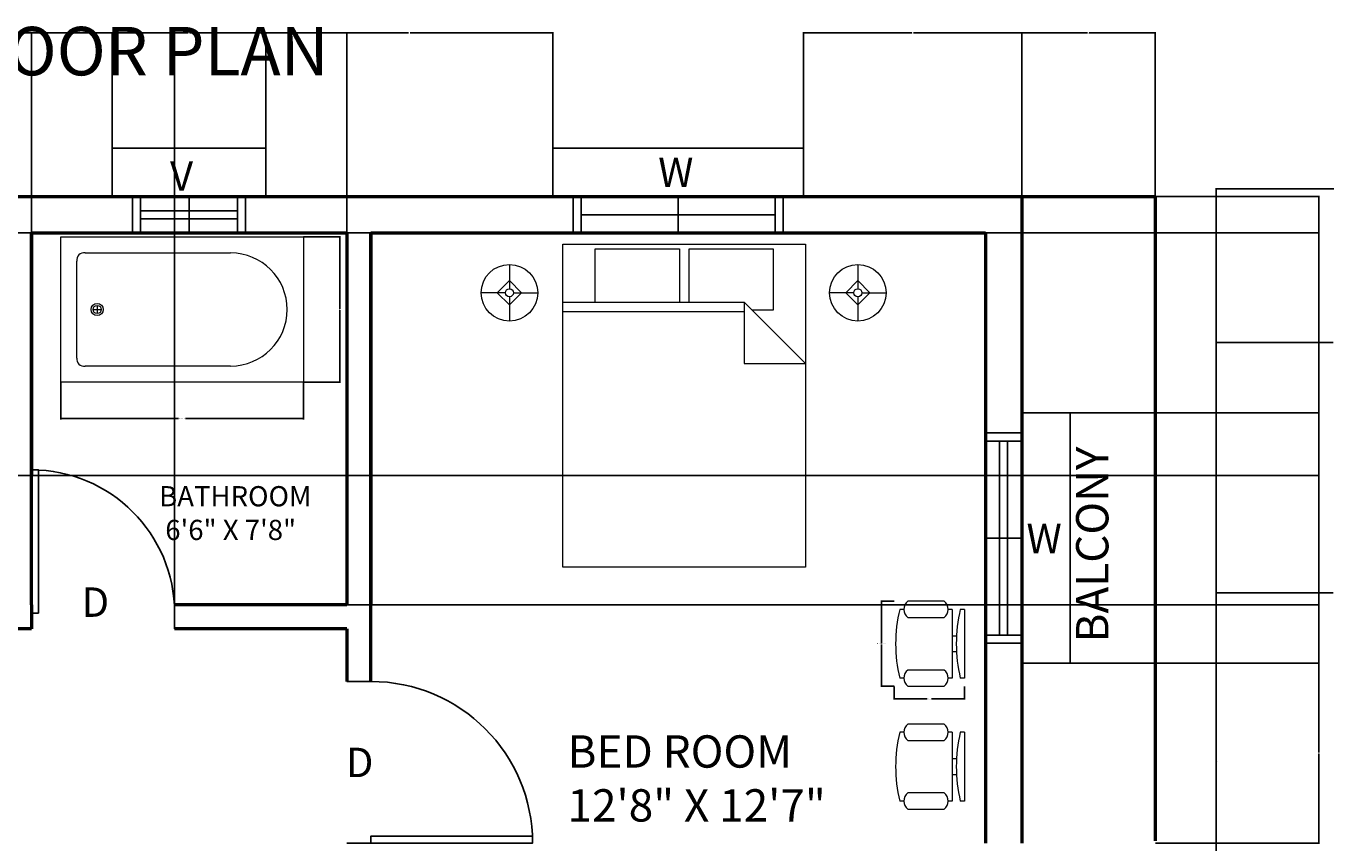
# Model space of a CAD drawing. Units: inches. Extents: x -73 to 1162, y -188 to 590.
# Tile 5 of 9: x 222 to 543, y -8 to 194. Entities that reach past the tile are written whole.
import ezdxf

# ---------------------------------------------------------------- set-up
doc = ezdxf.new("R2010")
doc.units = ezdxf.units.IN
doc.header["$MEASUREMENT"] = 0
for name, color, linetype, lineweight in [('A-ANNO-DIMS', 2, 'Continuous', 18), ('A-ANNO-TEXT', 7, 'Continuous', 25), ('A-AREA-IDEN', 2, 'Continuous', 25), ('A-DOOR', 3, 'Continuous', 25), ('A-FLOR-FIXT', 8, 'Continuous', 18), ('A-FURN', 8, 'Continuous', 18), ('A-GLAZ', 4, 'Continuous', 25), ('A-WALL', 7, 'Continuous', 50)]:
    doc.layers.add(name, color=color, linetype=linetype, lineweight=lineweight)
doc.styles.get("Standard").update_dxf_attribs({"font": 'arial.ttf'})
doc.dimstyles.get("Standard").update_dxf_attribs({"dimtxt": 0.18, "dimasz": 0.18, "dimexe": 0.18, "dimexo": 0.0625, "dimgap": 0.09, "dimtad": 0, "dimtih": 1, "dimtoh": 1, "dimdec": 1, "dimzin": 0, "dimdsep": 46, "dimlunit": 4, "dimtxsty": 'Standard', "dimcen": 0.09, "dimadec": 0, "dimazin": 0, "dimtfac": 1, "dimtdec": 1, "dimtofl": 0, "dimtmove": 0, "dimatfit": 3, "dimfxl": 1, "dimtolj": 1, "dimtzin": 0, "dimarcsym": 0})

# ---------------------------------------------------------------- blocks, each defined once
blk = doc.blocks.new('*U4')
for p, q in [((0, 0), (0, -100)), ((900, 0), (900, -100))]:
    blk.add_line(p, q)
blk.add_lwpolyline([(0, 0), (0, 900), (43.75, 900), (43.75, 0)], close=True)
blk.add_arc((0, 0), 900, 0, 90)
blk = doc.blocks.new('*U7')
for p, q in [((0, 0), (0, 6)), ((40, 0), (40, 6))]:
    blk.add_line(p, q)
blk.add_lwpolyline([(0, 0), (0, -40), (1.75, -40), (1.75, 0)], close=True)
blk.add_arc((0, 0), 40, 270, 360)
blk = doc.blocks.new('Bath Tub - 26 x 60 in.')
for p, q in [((8, -18), (10, -18)), ((9, -17), (9, -19))]:
    blk.add_line(p, q)
blk.add_lwpolyline([(0, -36), (0, 0), (60, 0), (60, -36)], close=True)
for points in [[(4, -30), (4, -6)], [(6, -4), (42, -4)], [(42, -32), (6, -32)]]:
    blk.add_lwpolyline(points)
for radius in [1.5, 1]:
    blk.add_circle((9, -18), radius)
for centre, radius, start, end in [((5.75, -5.75), 1.77, 81.8699, 188.1301), ((42, -18), 14, 270, 90), ((5.75, -30.25), 1.77, 171.8699, 278.1301)]:
    blk.add_arc(centre, radius, start, end)
blk = doc.blocks.new('Bed - Queen')
for p, q in [((0, -80.00003), (0, 0)), ((0, 0), (59.99999, 0)), ((59.99999, 0), (59.99999, -80.00003)), ((7.99999, -1.2), (28.79998, -1.2)), ((7.99999, -14.4), (7.99999, -1.2)), ((28.79998, -1.2), (28.79998, -14.4)), ((31.19999, -1.2), (51.99999, -1.2)), ((31.19999, -14.4), (31.19999, -1.2)), ((51.99999, -1.2), (51.99999, -16.4)), ((0, -14.4), (44.8, -14.4)), ((59.99999, -29.6), (44.8, -14.4)), ((44.8, -14.4), (44.8, -29.6)), ((44.8, -16.8), (0, -16.8)), ((51.99999, -16.4), (46.79936, -16.4)), ((44.8, -29.6), (59.99999, -29.6)), ((59.99999, -80.00003), (0, -80.00003))]:
    blk.add_line(p, q)
blk = doc.blocks.new('Lamp - Table')
for p, q in [((0, 7), (0, 1)), ((-1, 0), (-7, 0)), ((0, 3), (-3, 0)), ((-3, 0), (0, -3)), ((3, 0), (0, 3)), ((0, -3), (3, 0)), ((1, 0), (7, 0)), ((0, -1), (0, -7))]:
    blk.add_line(p, q)
for radius in [7, 1]:
    blk.add_circle((0, 0), radius)
blk = doc.blocks.new('Chair - Desk')
for p, q in [((-8.5, 0), (-8.5, -1)), ((-8.5, 0), (8.5, 0)), ((8.5, 0), (8.5, -1)), ((-8.5, -3), (-8.5, -4)), ((-8.5, -3), (8.5, -3)), ((-2, -3), (-2, -1.9355)), ((2, -1.9576), (2, -3)), ((8.5, -3), (8.5, -4)), ((-10.5, -5), (-10.5, -14)), ((-6.5, -14), (-6.5, -5)), ((6.5, -5), (6.5, -14)), ((10.5, -14), (10.5, -5)), ((-8.5, -15), (-8.5, -16)), ((8.5, -15), (8.5, -16))]:
    blk.add_line(p, q)
for centre, radius, start, end in [((0, 34.625), 36.625, 256.5803, 283.4197), ((-8.5, -6.5), 2.5, 36.8699, 143.1301), ((8.5, -6.5), 2.5, 36.8699, 143.1301), ((-8.5, -12.5), 2.5, 216.8699, 323.1301), ((0, 19.625), 36.625, 256.5803, 283.4197), ((8.5, -12.5), 2.5, 216.8699, 323.1301)]:
    blk.add_arc(centre, radius, start, end)
blk = doc.blocks.new('WIN-W')
for p, q in [((9, 57), (9, 62)), ((9, 62), (21, 62)), ((21, 62), (21, 0)), ((0, 57), (9, 57)), ((0, 5), (9, 5)), ((9, 5), (9, 0)), ((9, 0), (21, 0))]:
    blk.add_line(p, q)
blk = doc.blocks.new('VENT-V')
for p, q in [((0, 9), (0, 21)), ((38, 21), (0, 21)), ((38, 9), (38, 21)), ((5, 9), (0, 9)), ((5, 0), (5, 9)), ((33, 0), (33, 9)), ((33, 9), (38, 9))]:
    blk.add_line(p, q)
blk = doc.blocks.new('*D38')
at = {"layer": 'A-ANNO-DIMS', "color": 0, "lineweight": -2, "transparency": 16777216}
for p, q in [((436.58, 52.02), (433.32, 52.02)), ((433.5, 51.84), (433.5, 41.7)), ((433.5, 31.2), (433.5, 41.34)), ((436.58, 31.02), (433.32, 31.02))]:
    blk.add_line(p, q, dxfattribs=at)
at = {"layer": 'A-ANNO-DIMS', "color": 0, "transparency": 16777216}
for points in [[(433.47, 51.84), (433.53, 51.84), (433.5, 52.02)], [(433.47, 31.2), (433.53, 31.2), (433.5, 31.02)]]:
    blk.add_solid(points, dxfattribs=at)
at = {"layer": 'Defpoints', "color": 0, "transparency": 16777216}
for p in [(436.65, 52.02), (433.5, 31.02), (436.65, 31.02)]:
    blk.add_point(p, dxfattribs=at)
at = {"layer": 'A-ANNO-DIMS', "color": 0, "transparency": 16777216, "insert": (433.5, 41.52), "char_height": 0.18, "attachment_point": 5}
blk.add_mtext('\\A1;DESK CHAIR 21 TYP.', dxfattribs=at)
blk = doc.blocks.new('*D39')
at = {"layer": 'A-ANNO-DIMS', "color": 0, "lineweight": -2, "transparency": 16777216}
for p, q in [((436.65, 30.96), (436.65, 27.69)), ((453.98, 30.96), (453.98, 27.69)), ((436.83, 27.87), (444.79, 27.87)), ((453.8, 27.87), (445.83, 27.87))]:
    blk.add_line(p, q, dxfattribs=at)
at = {"layer": 'A-ANNO-DIMS', "color": 0, "transparency": 16777216}
for points in [[(436.83, 27.9), (436.83, 27.84), (436.65, 27.87)], [(453.8, 27.9), (453.8, 27.84), (453.98, 27.87)]]:
    blk.add_solid(points, dxfattribs=at)
at = {"layer": 'Defpoints', "color": 0, "transparency": 16777216}
for p in [(436.65, 31.02), (453.98, 31.02), (453.98, 27.87)]:
    blk.add_point(p, dxfattribs=at)
at = {"layer": 'A-ANNO-DIMS', "color": 0, "transparency": 16777216, "insert": (445.31, 27.87), "char_height": 0.18, "attachment_point": 5}
blk.add_mtext('\\A1;17 TYP.', dxfattribs=at)
blk = doc.blocks.new('*D52')
at = {"layer": 'A-ANNO-DIMS', "color": 0, "lineweight": -2, "transparency": 16777216}
for p, q in [((230.45, 106.17), (230.45, 97.05)), ((290.45, 106.17), (290.45, 97.05)), ((230.63, 97.23), (259.58, 97.23)), ((290.27, 97.23), (261.32, 97.23))]:
    blk.add_line(p, q, dxfattribs=at)
at = {"layer": 'A-ANNO-DIMS', "color": 0, "transparency": 16777216}
for points in [[(230.63, 97.26), (230.63, 97.2), (230.45, 97.23)], [(290.27, 97.26), (290.27, 97.2), (290.45, 97.23)]]:
    blk.add_solid(points, dxfattribs=at)
at = {"layer": 'Defpoints', "color": 0, "transparency": 16777216}
for p in [(230.45, 106.23), (290.45, 106.23), (290.45, 97.23)]:
    blk.add_point(p, dxfattribs=at)
at = {"layer": 'A-ANNO-DIMS', "color": 0, "transparency": 16777216, "insert": (260.45, 97.23), "char_height": 0.18, "attachment_point": 5}
blk.add_mtext('\\A1;BATH TUB 60', dxfattribs=at)
blk = doc.blocks.new('*D53')
at = {"layer": 'A-ANNO-DIMS', "color": 0, "lineweight": -2, "transparency": 16777216}
for p, q in [((290.51, 142.23), (299.63, 142.23)), ((299.45, 142.05), (299.45, 124.41)), ((299.45, 106.41), (299.45, 124.05)), ((290.51, 106.23), (299.63, 106.23))]:
    blk.add_line(p, q, dxfattribs=at)
at = {"layer": 'A-ANNO-DIMS', "color": 0, "transparency": 16777216}
for points in [[(299.42, 142.05), (299.48, 142.05), (299.45, 142.23)], [(299.42, 106.41), (299.48, 106.41), (299.45, 106.23)]]:
    blk.add_solid(points, dxfattribs=at)
at = {"layer": 'Defpoints', "color": 0, "transparency": 16777216}
for p in [(290.45, 142.23), (299.45, 142.23), (290.45, 106.23)]:
    blk.add_point(p, dxfattribs=at)
at = {"layer": 'A-ANNO-DIMS', "color": 0, "transparency": 16777216, "insert": (299.45, 124.23), "char_height": 0.18, "attachment_point": 5}
blk.add_mtext('\\A1;36', dxfattribs=at)
blk = doc.blocks.new('*D61')
at = {"layer": 'A-ANNO-DIMS', "color": 0, "lineweight": -2, "transparency": 16777216}
for p, q in [((197.17, 164.25), (197.17, 192.86)), ((197.35, 192.68), (219.95, 192.68)), ((242.99, 192.68), (220.39, 192.68)), ((243.17, 164.25), (243.17, 192.86))]:
    blk.add_line(p, q, dxfattribs=at)
at = {"layer": 'A-ANNO-DIMS', "color": 0, "transparency": 16777216}
for points in [[(197.35, 192.71), (197.35, 192.65), (197.17, 192.68)], [(242.99, 192.71), (242.99, 192.65), (243.17, 192.68)]]:
    blk.add_solid(points, dxfattribs=at)
at = {"layer": 'Defpoints', "color": 0, "transparency": 16777216}
for p in [(243.17, 192.68), (197.17, 164.18), (243.17, 164.18)]:
    blk.add_point(p, dxfattribs=at)
at = {"layer": 'A-ANNO-DIMS', "color": 0, "transparency": 16777216, "insert": (220.17, 192.68), "char_height": 0.18, "attachment_point": 5}
blk.add_mtext('\\A1;46', dxfattribs=at)
blk = doc.blocks.new('*D62')
at = {"layer": 'A-ANNO-DIMS', "color": 0, "lineweight": -2, "transparency": 16777216}
for p, q in [((281.17, 164.25), (281.17, 192.86)), ((281.35, 192.68), (316.47, 192.68)), ((351.99, 192.68), (316.87, 192.68)), ((352.17, 164.25), (352.17, 192.86))]:
    blk.add_line(p, q, dxfattribs=at)
at = {"layer": 'A-ANNO-DIMS', "color": 0, "transparency": 16777216}
for points in [[(281.35, 192.71), (281.35, 192.65), (281.17, 192.68)], [(351.99, 192.71), (351.99, 192.65), (352.17, 192.68)]]:
    blk.add_solid(points, dxfattribs=at)
at = {"layer": 'Defpoints', "color": 0, "transparency": 16777216}
for p in [(352.17, 192.68), (281.17, 164.18), (352.17, 164.18)]:
    blk.add_point(p, dxfattribs=at)
at = {"layer": 'A-ANNO-DIMS', "color": 0, "transparency": 16777216, "insert": (316.67, 192.68), "char_height": 0.18, "attachment_point": 5}
blk.add_mtext('\\A1;71', dxfattribs=at)
blk = doc.blocks.new('*D63')
at = {"layer": 'A-ANNO-DIMS', "color": 0, "lineweight": -2, "transparency": 16777216}
for p, q in [((414.17, 164.25), (414.17, 192.86)), ((414.35, 192.68), (440.95, 192.68)), ((467.99, 192.68), (441.39, 192.68)), ((468.17, 152.25), (468.17, 192.86))]:
    blk.add_line(p, q, dxfattribs=at)
at = {"layer": 'A-ANNO-DIMS', "color": 0, "transparency": 16777216}
for points in [[(414.35, 192.71), (414.35, 192.65), (414.17, 192.68)], [(467.99, 192.71), (467.99, 192.65), (468.17, 192.68)]]:
    blk.add_solid(points, dxfattribs=at)
at = {"layer": 'Defpoints', "color": 0, "transparency": 16777216}
for p in [(468.17, 192.68), (414.17, 164.18), (468.17, 152.18)]:
    blk.add_point(p, dxfattribs=at)
at = {"layer": 'A-ANNO-DIMS', "color": 0, "transparency": 16777216, "insert": (441.17, 192.68), "char_height": 0.18, "attachment_point": 5}
blk.add_mtext('\\A1;54', dxfattribs=at)
blk = doc.blocks.new('*D64')
at = {"layer": 'A-ANNO-DIMS', "color": 0, "lineweight": -2, "transparency": 16777216}
for p, q in [((468.17, 152.25), (468.17, 192.86)), ((468.35, 192.68), (484.45, 192.68)), ((500.99, 192.68), (484.89, 192.68)), ((501.17, 152.25), (501.17, 192.86))]:
    blk.add_line(p, q, dxfattribs=at)
at = {"layer": 'A-ANNO-DIMS', "color": 0, "transparency": 16777216}
for points in [[(468.35, 192.71), (468.35, 192.65), (468.17, 192.68)], [(500.99, 192.71), (500.99, 192.65), (501.17, 192.68)]]:
    blk.add_solid(points, dxfattribs=at)
at = {"layer": 'Defpoints', "color": 0, "transparency": 16777216}
for p in [(501.17, 192.68), (468.17, 152.18), (501.17, 152.18)]:
    blk.add_point(p, dxfattribs=at)
at = {"layer": 'A-ANNO-DIMS', "color": 0, "transparency": 16777216, "insert": (484.67, 192.68), "char_height": 0.18, "attachment_point": 5}
blk.add_mtext('\\A1;33', dxfattribs=at)
blk = doc.blocks.new('*D72')
at = {"layer": 'A-ANNO-DIMS', "color": 0, "lineweight": -2, "transparency": 16777216}
for p, q in [((501.23, 152.18), (541.85, 152.18)), ((541.67, 152), (541.67, 125.62)), ((541.67, 98.86), (541.67, 125.25)), ((480.23, 98.68), (541.85, 98.68))]:
    blk.add_line(p, q, dxfattribs=at)
at = {"layer": 'A-ANNO-DIMS', "color": 0, "transparency": 16777216}
for points in [[(541.64, 152), (541.7, 152), (541.67, 152.18)], [(541.64, 98.86), (541.7, 98.86), (541.67, 98.68)]]:
    blk.add_solid(points, dxfattribs=at)
at = {"layer": 'Defpoints', "color": 0, "transparency": 16777216}
for p in [(501.17, 152.18), (480.17, 98.68), (541.67, 98.68)]:
    blk.add_point(p, dxfattribs=at)
at = {"layer": 'A-ANNO-DIMS', "color": 0, "transparency": 16777216, "insert": (541.67, 125.43), "char_height": 0.18, "attachment_point": 5}
blk.add_mtext('\\A1;53.5', dxfattribs=at)
blk = doc.blocks.new('*D73')
at = {"layer": 'A-ANNO-DIMS', "color": 0, "lineweight": -2, "transparency": 16777216}
for p, q in [((480.23, 98.68), (541.85, 98.68)), ((541.67, 98.5), (541.67, 67.87)), ((541.67, 36.86), (541.67, 67.5)), ((480.23, 36.68), (541.85, 36.68))]:
    blk.add_line(p, q, dxfattribs=at)
at = {"layer": 'A-ANNO-DIMS', "color": 0, "transparency": 16777216}
for points in [[(541.64, 98.5), (541.7, 98.5), (541.67, 98.68)], [(541.64, 36.86), (541.7, 36.86), (541.67, 36.68)]]:
    blk.add_solid(points, dxfattribs=at)
at = {"layer": 'Defpoints', "color": 0, "transparency": 16777216}
for p in [(480.17, 98.68), (480.17, 36.68), (541.67, 36.68)]:
    blk.add_point(p, dxfattribs=at)
at = {"layer": 'A-ANNO-DIMS', "color": 0, "transparency": 16777216, "insert": (541.67, 67.68), "char_height": 0.18, "attachment_point": 5}
blk.add_mtext('\\A1;62', dxfattribs=at)
blk = doc.blocks.new('*D74')
at = {"layer": 'A-ANNO-DIMS', "color": 0, "lineweight": -2, "transparency": 16777216}
for p, q in [((480.23, 36.68), (541.85, 36.68)), ((541.67, 36.5), (541.67, 14.62)), ((541.67, -7.64), (541.67, 14.25)), ((501.23, -7.82), (541.85, -7.82))]:
    blk.add_line(p, q, dxfattribs=at)
at = {"layer": 'A-ANNO-DIMS', "color": 0, "transparency": 16777216}
for points in [[(541.64, 36.5), (541.7, 36.5), (541.67, 36.68)], [(541.64, -7.64), (541.7, -7.64), (541.67, -7.82)]]:
    blk.add_solid(points, dxfattribs=at)
at = {"layer": 'Defpoints', "color": 0, "transparency": 16777216}
for p in [(480.17, 36.68), (501.17, -7.82), (541.67, -7.82)]:
    blk.add_point(p, dxfattribs=at)
at = {"layer": 'A-ANNO-DIMS', "color": 0, "transparency": 16777216, "insert": (541.67, 14.43), "char_height": 0.18, "attachment_point": 5}
blk.add_mtext('\\A1;44.5', dxfattribs=at)
blk = doc.blocks.new('*D90')
at = {"layer": 'A-ANNO-DIMS', "color": 0, "lineweight": -2, "transparency": 16777216}
for p, q in [((217.17, 143.25), (217.17, 192.86)), ((217.35, 192.68), (220.02, 192.68)), ((222.99, 192.68), (220.32, 192.68)), ((223.17, 143.25), (223.17, 192.86))]:
    blk.add_line(p, q, dxfattribs=at)
at = {"layer": 'A-ANNO-DIMS', "color": 0, "transparency": 16777216}
for points in [[(217.35, 192.71), (217.35, 192.65), (217.17, 192.68)], [(222.99, 192.71), (222.99, 192.65), (223.17, 192.68)]]:
    blk.add_solid(points, dxfattribs=at)
at = {"layer": 'Defpoints', "color": 0, "transparency": 16777216}
for p in [(223.17, 192.68), (217.17, 143.18), (223.17, 143.18)]:
    blk.add_point(p, dxfattribs=at)
at = {"layer": 'A-ANNO-DIMS', "color": 0, "transparency": 16777216, "insert": (220.17, 192.68), "char_height": 0.18, "attachment_point": 5}
blk.add_mtext('\\A1;6', dxfattribs=at)
blk = doc.blocks.new('*D91')
at = {"layer": 'A-ANNO-DIMS', "color": 0, "lineweight": -2, "transparency": 16777216}
for p, q in [((223.17, 143.25), (223.17, 192.86)), ((223.35, 192.68), (261.95, 192.68)), ((300.99, 192.68), (262.39, 192.68)), ((301.17, 143.25), (301.17, 192.86))]:
    blk.add_line(p, q, dxfattribs=at)
at = {"layer": 'A-ANNO-DIMS', "color": 0, "transparency": 16777216}
for points in [[(223.35, 192.71), (223.35, 192.65), (223.17, 192.68)], [(300.99, 192.71), (300.99, 192.65), (301.17, 192.68)]]:
    blk.add_solid(points, dxfattribs=at)
at = {"layer": 'Defpoints', "color": 0, "transparency": 16777216}
for p in [(301.17, 192.68), (223.17, 143.18), (301.17, 143.18)]:
    blk.add_point(p, dxfattribs=at)
at = {"layer": 'A-ANNO-DIMS', "color": 0, "transparency": 16777216, "insert": (262.17, 192.68), "char_height": 0.18, "attachment_point": 5}
blk.add_mtext('\\A1;78', dxfattribs=at)
blk = doc.blocks.new('*D93')
at = {"layer": 'A-ANNO-DIMS', "color": 0, "lineweight": -2, "transparency": 16777216}
for p, q in [((139.23, 143.18), (541.85, 143.18)), ((541.67, 143), (541.67, 113.37)), ((541.67, 83.36), (541.67, 113)), ((139.23, 83.18), (541.85, 83.18))]:
    blk.add_line(p, q, dxfattribs=at)
at = {"layer": 'A-ANNO-DIMS', "color": 0, "transparency": 16777216}
for points in [[(541.64, 143), (541.7, 143), (541.67, 143.18)], [(541.64, 83.36), (541.7, 83.36), (541.67, 83.18)]]:
    blk.add_solid(points, dxfattribs=at)
at = {"layer": 'Defpoints', "color": 0, "transparency": 16777216}
for p in [(139.17, 143.18), (139.17, 83.18), (541.67, 83.18)]:
    blk.add_point(p, dxfattribs=at)
at = {"layer": 'A-ANNO-DIMS', "color": 0, "transparency": 16777216, "insert": (541.67, 113.18), "char_height": 0.18, "attachment_point": 5}
blk.add_mtext('\\A1;60', dxfattribs=at)
blk = doc.blocks.new('*D94')
at = {"layer": 'A-ANNO-DIMS', "color": 0, "lineweight": -2, "transparency": 16777216}
for p, q in [((301.23, 143.18), (541.85, 143.18)), ((541.67, 143), (541.67, 97.37)), ((541.67, 51.36), (541.67, 97)), ((301.23, 51.18), (541.85, 51.18))]:
    blk.add_line(p, q, dxfattribs=at)
at = {"layer": 'A-ANNO-DIMS', "color": 0, "transparency": 16777216}
for points in [[(541.64, 143), (541.7, 143), (541.67, 143.18)], [(541.64, 51.36), (541.7, 51.36), (541.67, 51.18)]]:
    blk.add_solid(points, dxfattribs=at)
at = {"layer": 'Defpoints', "color": 0, "transparency": 16777216}
for p in [(301.17, 143.18), (301.17, 51.18), (541.67, 51.18)]:
    blk.add_point(p, dxfattribs=at)
at = {"layer": 'A-ANNO-DIMS', "color": 0, "transparency": 16777216, "insert": (541.67, 97.18), "char_height": 0.18, "attachment_point": 5}
blk.add_mtext('\\A1;92', dxfattribs=at)
blk = doc.blocks.new('*D97')
at = {"layer": 'A-ANNO-DIMS', "color": 0, "lineweight": -2, "transparency": 16777216}
for p, q in [((223.17, 51.25), (223.17, 192.86)), ((223.35, 192.68), (240.49, 192.68)), ((258.42, 192.68), (241.28, 192.68)), ((258.6, 51.25), (258.6, 192.86))]:
    blk.add_line(p, q, dxfattribs=at)
at = {"layer": 'A-ANNO-DIMS', "color": 0, "transparency": 16777216}
for points in [[(223.35, 192.71), (223.35, 192.65), (223.17, 192.68)], [(258.42, 192.71), (258.42, 192.65), (258.6, 192.68)]]:
    blk.add_solid(points, dxfattribs=at)
at = {"layer": 'Defpoints', "color": 0, "transparency": 16777216}
for p in [(258.6, 192.68), (223.17, 51.18), (258.6, 51.18)]:
    blk.add_point(p, dxfattribs=at)
at = {"layer": 'A-ANNO-DIMS', "color": 0, "transparency": 16777216, "insert": (240.89, 192.68), "char_height": 0.18, "attachment_point": 5}
blk.add_mtext('\\A1;35.43', dxfattribs=at)
blk = doc.blocks.new('*D104')
at = {"layer": 'A-ANNO-DIMS', "color": 0, "lineweight": -2, "transparency": 16777216}
for p, q in [((557.24, 154.09), (516.13, 154.09)), ((516.31, 153.91), (516.31, 4.27)), ((516.31, -145.73), (516.31, 3.91)), ((557.24, -145.91), (516.13, -145.91))]:
    blk.add_line(p, q, dxfattribs=at)
at = {"layer": 'A-ANNO-DIMS', "color": 0, "transparency": 16777216}
for points in [[(516.28, 153.91), (516.34, 153.91), (516.31, 154.09)], [(516.28, -145.73), (516.34, -145.73), (516.31, -145.91)]]:
    blk.add_solid(points, dxfattribs=at)
at = {"layer": 'Defpoints', "color": 0, "transparency": 16777216}
for p in [(557.31, 154.09), (516.31, -145.91), (557.31, -145.91)]:
    blk.add_point(p, dxfattribs=at)
at = {"layer": 'A-ANNO-DIMS', "color": 0, "transparency": 16777216, "insert": (516.31, 4.09), "char_height": 0.18, "attachment_point": 5}
blk.add_mtext('\\A1;300', dxfattribs=at)
blk = doc.blocks.new('*D105')
at = {"layer": 'A-ANNO-DIMS', "color": 0, "lineweight": -2, "transparency": 16777216}
for p, q in [((557.24, 154.09), (516.13, 154.09)), ((516.31, 153.91), (516.31, 135.27)), ((516.31, 116.27), (516.31, 134.91)), ((545.24, 116.09), (516.13, 116.09))]:
    blk.add_line(p, q, dxfattribs=at)
at = {"layer": 'A-ANNO-DIMS', "color": 0, "transparency": 16777216}
for points in [[(516.28, 153.91), (516.34, 153.91), (516.31, 154.09)], [(516.28, 116.27), (516.34, 116.27), (516.31, 116.09)]]:
    blk.add_solid(points, dxfattribs=at)
at = {"layer": 'Defpoints', "color": 0, "transparency": 16777216}
for p in [(557.31, 154.09), (516.31, 116.09), (545.31, 116.09)]:
    blk.add_point(p, dxfattribs=at)
at = {"layer": 'A-ANNO-DIMS', "color": 0, "transparency": 16777216, "insert": (516.31, 135.09), "char_height": 0.18, "attachment_point": 5}
blk.add_mtext('\\A1;38', dxfattribs=at)
blk = doc.blocks.new('*D106')
at = {"layer": 'A-ANNO-DIMS', "color": 0, "lineweight": -2, "transparency": 16777216}
for p, q in [((545.24, 54.09), (516.13, 54.09)), ((516.31, 53.91), (516.31, 12.52)), ((516.31, -29.23), (516.31, 12.16)), ((545.24, -29.41), (516.13, -29.41))]:
    blk.add_line(p, q, dxfattribs=at)
at = {"layer": 'A-ANNO-DIMS', "color": 0, "transparency": 16777216}
for points in [[(516.28, 53.91), (516.34, 53.91), (516.31, 54.09)], [(516.28, -29.23), (516.34, -29.23), (516.31, -29.41)]]:
    blk.add_solid(points, dxfattribs=at)
at = {"layer": 'Defpoints', "color": 0, "transparency": 16777216}
for p in [(545.31, 54.09), (516.31, -29.41), (545.31, -29.41)]:
    blk.add_point(p, dxfattribs=at)
at = {"layer": 'A-ANNO-DIMS', "color": 0, "transparency": 16777216, "insert": (516.31, 12.34), "char_height": 0.18, "attachment_point": 5}
blk.add_mtext('\\A1;83.5', dxfattribs=at)

msp = doc.modelspace()

# ---------------------------------------------------------------- linework, layer by layer
at = {"layer": 'A-GLAZ'}
for p, q in [((250.17, 143.1844), (250.17, 152.1844)), ((262.17, 143.1844), (262.17, 152.1844)), ((274.17, 143.1844), (274.17, 152.1844)), ((359.17, 143.1844), (359.17, 152.1844)), ((383.17, 143.1844), (383.17, 152.1844)), ((407.17, 143.1844), (407.17, 152.1844)), ((250.17, 148.6844), (274.17, 148.6844)), ((250.17, 146.6844), (274.17, 146.6844)), ((359.17, 147.6844), (407.17, 147.6844)), ((459.17, 91.6844), (468.17, 91.6844)), ((462.67, 91.6844), (462.67, 43.6844)), ((464.67, 91.6844), (464.67, 43.6844)), ((459.17, 67.6844), (468.17, 67.6844)), ((459.17, 43.6844), (468.17, 43.6844))]:
    msp.add_line(p, q, dxfattribs=at)
at = {"layer": 'A-WALL'}
for p, q in [((139.17, 152.1844), (223.17, 152.1844)), ((223.17, 152.1844), (307.17, 152.1844)), ((307.17, 152.1844), (459.17, 152.1844)), ((459.17, 152.1844), (483.17, 152.1844)), ((468.17, 152.1844), (468.17, -7.8156)), ((483.17, 152.1844), (492.17, 152.1844)), ((492.17, 152.1844), (501.17, 152.1844)), ((501.17, 152.1844), (501.17, -7.2633)), ((223.17, 143.1844), (223.17, 83.1844)), ((223.17, 143.1844), (301.17, 143.1844)), ((223.17, 51.1844), (223.17, 143.1844)), ((301.17, 143.1844), (301.17, 51.1844)), ((307.17, 143.1844), (307.17, 51.1844)), ((307.17, 143.1844), (459.17, 143.1844)), ((307.17, 32.1844), (307.17, 143.1844)), ((459.17, 143.1844), (459.17, -7.8156)), ((223.17, 51.1844), (223.17, 45.1844)), ((301.17, 51.1844), (258.6031, 51.1844)), ((223.17, 45.1844), (217.17, 45.1844)), ((301.17, 45.1844), (258.6031, 45.1844)), ((301.17, 45.1844), (301.17, 32.1844))]:
    msp.add_line(p, q, dxfattribs=at)

# ---------------------------------------------------------------- block references
at = {"layer": 'A-DOOR', "xscale": 0.0393700787401575, "yscale": 0.0393700787401575, "zscale": 0.0393700787401575}
msp.add_blockref('*U4', (223.17, 49.1215), dxfattribs=at)
at = {"layer": 'A-DOOR', "rotation": 90}
msp.add_blockref('*U7', (307.17, -7.8156), dxfattribs=at)
at = {"layer": 'A-FLOR-FIXT'}
msp.add_blockref('Bath Tub - 26 x 60 in.', (230.4497, 142.2293), dxfattribs=at)
at = {"layer": 'A-FURN'}
for name, p in [('Bed - Queen', (354.6764, 140.4332)), ('Lamp - Table', (341.4413, 128.374)), ('Lamp - Table', (427.6218, 128.374))]:
    msp.add_blockref(name, p, dxfattribs=at)
at = {"layer": 'A-FURN', "rotation": 270}
for p in [(453.9792, 41.5197), (453.9792, 11.1043)]:
    msp.add_blockref('Chair - Desk', p, dxfattribs=at)
at = {"layer": 'A-GLAZ'}
for name, p in [('VENT-V', (243.17, 143.184)), ('WIN-W', (459.17, 36.684))]:
    msp.add_blockref(name, p, dxfattribs=at)
at = {"layer": 'A-GLAZ', "rotation": 90.00000000000006}
msp.add_blockref('WIN-W', (414.1704, 143.1844), dxfattribs=at)

# ---------------------------------------------------------------- texts
at = {"layer": 'A-ANNO-TEXT'}
for s, p in [('V', (257.4666, 153.645)), ('W', (378.2297, 154.5576)), ('W', (469.3502, 63.9253)), ('D', (235.5792, 48.174)), ('D', (300.9504, 8.5138))]:
    msp.add_text(s, height=7.2829, dxfattribs=at).set_placement(p)
at = {"layer": 'A-ANNO-TEXT', "insert": (126.968, 194.1746), "char_height": 12, "attachment_point": 1}
msp.add_mtext_dynamic_manual_height_columns('GROUND FLOOR PLAN', width=198.609453, gutter_width=1, heights=[0], dxfattribs=at)
at = {"layer": 'A-AREA-IDEN', "insert": (481.6193, 41.8284), "char_height": 8, "attachment_point": 1, "rotation": 90}
msp.add_mtext_dynamic_manual_height_columns('BALCONY', width=71.534965, gutter_width=1, heights=[0], dxfattribs=at)
at = {"layer": 'A-AREA-IDEN', "attachment_point": 1}
for s, insert, char_height in [('BATHROOM\\P 6\'6" X 7\'8"', (254.7677, 80.5239), 5), ('BED ROOM\\P12\'8" X 12\'7"', (355.7974, 18.8595), 8)]:
    msp.add_mtext_dynamic_manual_height_columns(s, width=71.534965, gutter_width=1, heights=[0], dxfattribs=dict(at, insert=insert, char_height=char_height))

# ---------------------------------------------------------------- dimensions: what is measured, and where the dimension line sits
at = {"layer": 'A-ANNO-DIMS'}
for base, p1, p2, override, picture, middle in [((243.17, 192.6844), (197.17, 164.1844), (243.17, 164.1844), {"dimdec": 0, "dimlfac": 1, "dimrnd": 0, "dimzin": 0, "dimdsep": 46, "dimlunit": 2}, '*D61', (220.17, 192.6844)), ((223.17, 192.6844), (217.17, 143.1844), (223.17, 143.1844), {"dimdec": 0, "dimlfac": 1, "dimrnd": 0, "dimzin": 0, "dimdsep": 46, "dimlunit": 2}, '*D90', (220.17, 192.6844)), ((301.17, 192.6844), (223.17, 143.1844), (301.17, 143.1844), {"dimdec": 0, "dimlfac": 1, "dimrnd": 0, "dimzin": 0, "dimdsep": 46, "dimlunit": 2}, '*D91', (262.17, 192.6844)), ((258.6031, 192.6844), (223.17, 51.1844), (258.6031, 51.1844), {"dimdec": 2, "dimlfac": 1, "dimrnd": 0, "dimzin": 0, "dimdsep": 46, "dimlunit": 2}, '*D97', (240.8865, 192.6844)), ((352.17, 192.6844), (281.17, 164.1844), (352.17, 164.1844), {"dimdec": 0, "dimlfac": 1, "dimrnd": 0, "dimzin": 0, "dimdsep": 46, "dimlunit": 2}, '*D62', (316.67, 192.6844)), ((468.17, 192.6844), (414.17, 164.1844), (468.17, 152.1844), {"dimdec": 0, "dimlfac": 1, "dimrnd": 0, "dimzin": 0, "dimdsep": 46, "dimlunit": 2}, '*D63', (441.17, 192.6844)), ((501.17, 192.6844), (468.17, 152.1844), (501.17, 152.1844), {"dimdec": 0, "dimlfac": 1, "dimrnd": 0, "dimzin": 0, "dimdsep": 46, "dimlunit": 2}, '*D64', (484.67, 192.6844))]:
    dim = msp.add_linear_dim(base=base, p1=p1, p2=p2, dimstyle='Standard', override=override, dxfattribs=at)
    dim.commit()
    dim.dimension.update_dxf_attribs({"geometry": picture, "text_midpoint": middle})
for base, p1, p2, override, picture, middle in [((541.67, 98.6844), (501.17, 152.1844), (480.17, 98.6844), {"dimdec": 1, "dimlfac": 1, "dimrnd": 0, "dimzin": 0, "dimdsep": 46, "dimlunit": 2}, '*D72', (541.67, 125.4344)), ((516.307, -145.9077), (557.307, 154.0923), (557.307, -145.9077), {"dimdec": 0, "dimlfac": 1, "dimrnd": 0, "dimzin": 0, "dimdsep": 46, "dimlunit": 2}, '*D104', (516.307, 4.0923)), ((516.307, 116.0923), (557.307, 154.0923), (545.307, 116.0923), {"dimdec": 0, "dimlfac": 1, "dimrnd": 0, "dimzin": 0, "dimdsep": 46, "dimlunit": 2}, '*D105', (516.307, 135.0923)), ((541.67, 83.1844), (139.17, 143.1844), (139.17, 83.1844), {"dimdec": 0, "dimlfac": 1, "dimrnd": 0, "dimzin": 0, "dimdsep": 46, "dimlunit": 2}, '*D93', (541.67, 113.1844)), ((299.4497, 142.2293), (290.4497, 106.2293), (290.4497, 142.2293), {"dimdec": 0, "dimrnd": 0, "dimzin": 0, "dimlunit": 2}, '*D53', (299.4497, 124.2293)), ((541.67, 51.1844), (301.17, 143.1844), (301.17, 51.1844), {"dimdec": 0, "dimlfac": 1, "dimrnd": 0, "dimzin": 0, "dimdsep": 46, "dimlunit": 2}, '*D94', (541.67, 97.1844)), ((541.67, 36.6844), (480.17, 98.6844), (480.17, 36.6844), {"dimdec": 0, "dimlfac": 1, "dimrnd": 0, "dimzin": 0, "dimdsep": 46, "dimlunit": 2}, '*D73', (541.67, 67.6844)), ((516.307, -29.4077), (545.307, 54.0923), (545.307, -29.4077), {"dimdec": 1, "dimlfac": 1, "dimrnd": 0, "dimzin": 0, "dimdsep": 46, "dimlunit": 2}, '*D106', (516.307, 12.3423)), ((541.67, -7.8156), (480.17, 36.6844), (501.17, -7.8156), {"dimdec": 1, "dimlfac": 1, "dimrnd": 0, "dimzin": 0, "dimdsep": 46, "dimlunit": 2}, '*D74', (541.67, 14.4344))]:
    dim = msp.add_linear_dim(base=base, p1=p1, p2=p2, angle=90, dimstyle='Standard', override=override, dxfattribs=at)
    dim.commit()
    dim.dimension.update_dxf_attribs({"geometry": picture, "text_midpoint": middle})
for base, p1, p2, text, picture, middle in [((290.4497, 97.2293), (230.4497, 106.2293), (290.4497, 106.2293), 'BATH TUB <>', '*D52', (260.4497, 97.2293)), ((453.9792, 27.8697), (436.6458, 31.0197), (453.9792, 31.0197), '<> TYP.', '*D39', (445.3125, 27.8697))]:
    dim = msp.add_linear_dim(base=base, p1=p1, p2=p2, text=text, dimstyle='Standard', override={"dimdec": 0, "dimrnd": 0, "dimzin": 0, "dimlunit": 2}, dxfattribs=at)
    dim.commit()
    dim.dimension.update_dxf_attribs({"geometry": picture, "text_midpoint": middle})
dim = msp.add_linear_dim(base=(433.4958, 31.0197), p1=(436.6458, 52.0197), p2=(436.6458, 31.0197), angle=270, text='DESK CHAIR <> TYP.', dimstyle='Standard', override={"dimdec": 0, "dimrnd": 0, "dimzin": 0, "dimlunit": 2}, dxfattribs=at)
dim.commit()
dim.dimension.update_dxf_attribs({"geometry": '*D38', "text_midpoint": (433.4958, 41.5197)})

doc.saveas('drawing.dxf')
